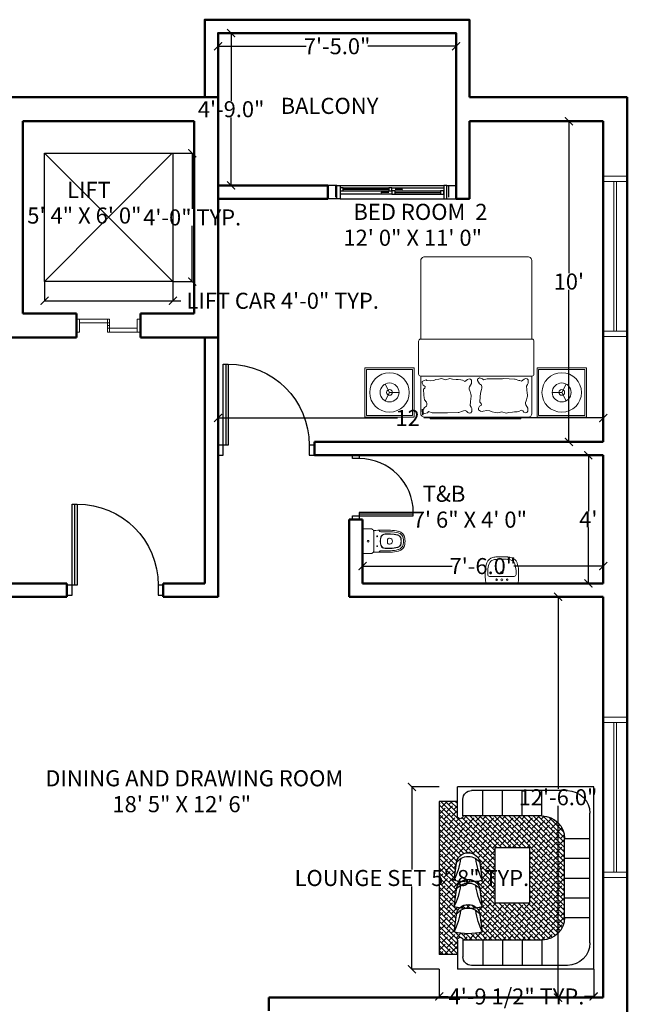
# Model space of a CAD drawing. Units: inches. Extents: x 147 to 1638, y 107 to 941.
# Tile 17 of 17: x 1368 to 1595, y 570 to 939. Entities that reach past the tile are written whole.
import ezdxf

# ---------------------------------------------------------------- set-up
doc = ezdxf.new("R2010")
doc.units = ezdxf.units.IN
doc.header["$MEASUREMENT"] = 0
for name, color, linetype, lineweight in [('A-ANNO-DIMS', 2, 'Continuous', 15), ('A-AREA-IDEN', 7, 'Continuous', 18), ('A-Door', 150, 'Continuous', 25), ('A-EQPM-ELEV', 7, 'Continuous', 25), ('A-FLOR-FIXT', 9, 'Continuous', 18), ('furniture', 50, 'Continuous', 18), ('HAT', 9, 'Continuous', 0), ('lift door', 200, 'Continuous', 20), ('walls', 7, 'Continuous', 50), ('windows', 3, 'Continuous', 20)]:
    doc.layers.add(name, color=color, linetype=linetype, lineweight=lineweight)
for name, color, linetype in [('A-Glaz', 92, 'Continuous'), ('FUR', 42, 'Continuous'), ('NT', 1, 'Continuous'), ('Win', 152, 'Continuous')]:
    doc.layers.add(name, color=color, linetype=linetype)
doc.styles.get("Standard").update_dxf_attribs({"font": 'arial.ttf'})
doc.dimstyles.get("Standard").update_dxf_attribs({"dimtxt": 6, "dimasz": 3, "dimexe": 0.18, "dimexo": 0.0625, "dimgap": 0.09, "dimtad": 0, "dimtih": 1, "dimtoh": 1, "dimdec": 1, "dimzin": 0, "dimdsep": 46, "dimlunit": 3, "dimtxsty": 'Standard', "dimblk": 'ARCHTICK', "dimcen": 0.09, "dimadec": 0, "dimazin": 0, "dimtfac": 1, "dimtdec": 1, "dimtofl": 0, "dimtmove": 0, "dimatfit": 3, "dimfxl": 1, "dimtolj": 1, "dimtzin": 0, "dimarcsym": 0})

# ---------------------------------------------------------------- blocks, each defined once
blk = doc.blocks.new('A$C087A3AA9')
at = {"layer": 'A-Door'}
for points in [[(852.6, 94.7), (852.6, 852.6), (805.3, 852.6), (805.3, 94.7)], [(47.4, 94.7), (47.4, 0), (0, 0), (0, 94.7)], [(900, 94.7), (900, 0), (852.6, 0), (852.6, 94.7)]]:
    blk.add_lwpolyline(points, close=True, dxfattribs=at)
at = {"layer": 'A-Glaz'}
blk.add_line((828.9, 852.6), (828.9, 94.7), dxfattribs=at)
at = {"layer": 'NT'}
blk.add_arc((805.3, 94.7), 757.9, 90, 180, dxfattribs=at)
blk = doc.blocks.new('_ArchTick')
at = {"color": 0, "linetype": 'ByBlock', "const_width": 0.15}
blk.add_lwpolyline([(-0.5, -0.5), (0.5, 0.5)], dxfattribs=at)
blk = doc.blocks.new('*D44')
at = {"layer": 'A-ANNO-DIMS', "color": 0, "lineweight": -2, "transparency": 16777216}
for p, q in [((1576.66, 722.72), (1568.7, 722.72)), ((1568.88, 722.72), (1568.88, 650.87)), ((1568.88, 572.72), (1568.88, 644.56)), ((1576.66, 572.72), (1568.7, 572.72))]:
    blk.add_line(p, q, dxfattribs=at)
at = {"layer": 'Defpoints', "color": 0, "lineweight": -2, "transparency": 16777216}
for p in [(1576.72, 722.72), (1568.88, 572.72), (1576.72, 572.72)]:
    blk.add_point(p, dxfattribs=at)
at = {"layer": 'A-ANNO-DIMS', "color": 0, "lineweight": -2, "transparency": 16777216, "xscale": 3, "yscale": 3, "zscale": 3}
for p, rotation in [((1568.88, 722.72), 90), ((1568.88, 572.72), 270)]:
    blk.add_blockref('_ArchTick', p, dxfattribs=dict(at, rotation=rotation))
at = {"layer": 'A-ANNO-DIMS', "color": 0, "transparency": 16777216, "insert": (1568.88, 647.72), "char_height": 6, "attachment_point": 5}
blk.add_mtext('\\A1;12\'-6.0"', dxfattribs=at)
blk = doc.blocks.new('*D45')
at = {"layer": 'A-ANNO-DIMS', "color": 0, "lineweight": -2, "transparency": 16777216}
for p, q in [((1566.15, 775.72), (1580.39, 775.72)), ((1580.21, 775.72), (1580.21, 754.81)), ((1580.21, 727.72), (1580.21, 748.63)), ((1566.15, 727.72), (1580.39, 727.72))]:
    blk.add_line(p, q, dxfattribs=at)
at = {"layer": 'Defpoints', "color": 0, "lineweight": -2, "transparency": 16777216}
for p in [(1566.09, 775.72), (1566.09, 727.72), (1580.21, 727.72)]:
    blk.add_point(p, dxfattribs=at)
at = {"layer": 'A-ANNO-DIMS', "color": 0, "lineweight": -2, "transparency": 16777216, "xscale": 3, "yscale": 3, "zscale": 3}
for p, rotation in [((1580.21, 775.72), 90), ((1580.21, 727.72), 270)]:
    blk.add_blockref('_ArchTick', p, dxfattribs=dict(at, rotation=rotation))
at = {"layer": 'A-ANNO-DIMS', "color": 0, "transparency": 16777216, "insert": (1580.21, 751.72), "char_height": 6, "attachment_point": 5}
blk.add_mtext("\\A1;4'", dxfattribs=at)
blk = doc.blocks.new('*D46')
at = {"layer": 'A-ANNO-DIMS', "color": 0, "lineweight": -2, "transparency": 16777216}
for p, q in [((1495.77, 730.37), (1495.77, 734.4)), ((1495.77, 734.22), (1529.23, 734.22)), ((1585.77, 734.22), (1552.3, 734.22)), ((1585.77, 730.37), (1585.77, 734.4))]:
    blk.add_line(p, q, dxfattribs=at)
at = {"layer": 'Defpoints', "color": 0, "lineweight": -2, "transparency": 16777216}
for p in [(1585.77, 734.22), (1495.77, 730.3), (1585.77, 730.3)]:
    blk.add_point(p, dxfattribs=at)
at = {"layer": 'A-ANNO-DIMS', "color": 0, "lineweight": -2, "transparency": 16777216, "xscale": 3, "yscale": 3, "zscale": 3, "rotation": 180}
blk.add_blockref('_ArchTick', (1495.77, 734.22), dxfattribs=at)
at = {"layer": 'A-ANNO-DIMS', "color": 0, "lineweight": -2, "transparency": 16777216, "xscale": 3, "yscale": 3, "zscale": 3}
blk.add_blockref('_ArchTick', (1585.77, 734.22), dxfattribs=at)
at = {"layer": 'A-ANNO-DIMS', "color": 0, "transparency": 16777216, "insert": (1540.77, 734.22), "char_height": 6, "attachment_point": 5}
blk.add_mtext('\\A1;7\'-6.0"', dxfattribs=at)
blk = doc.blocks.new('*D47')
at = {"layer": 'A-ANNO-DIMS', "color": 0, "lineweight": -2, "transparency": 16777216}
for p, q in [((1441.77, 785.96), (1441.77, 789.84)), ((1441.77, 789.66), (1508.87, 789.66)), ((1585.77, 789.66), (1518.67, 789.66)), ((1585.77, 785.96), (1585.77, 789.84))]:
    blk.add_line(p, q, dxfattribs=at)
at = {"layer": 'Defpoints', "color": 0, "lineweight": -2, "transparency": 16777216}
for p in [(1585.77, 789.66), (1441.77, 785.9), (1585.77, 785.9)]:
    blk.add_point(p, dxfattribs=at)
at = {"layer": 'A-ANNO-DIMS', "color": 0, "lineweight": -2, "transparency": 16777216, "xscale": 3, "yscale": 3, "zscale": 3, "rotation": 180}
blk.add_blockref('_ArchTick', (1441.77, 789.66), dxfattribs=at)
at = {"layer": 'A-ANNO-DIMS', "color": 0, "lineweight": -2, "transparency": 16777216, "xscale": 3, "yscale": 3, "zscale": 3}
blk.add_blockref('_ArchTick', (1585.77, 789.66), dxfattribs=at)
at = {"layer": 'A-ANNO-DIMS', "color": 0, "transparency": 16777216, "insert": (1513.77, 789.66), "char_height": 6, "attachment_point": 5}
blk.add_mtext("\\A1;12'", dxfattribs=at)
blk = doc.blocks.new('*D48')
at = {"layer": 'A-ANNO-DIMS', "color": 0, "lineweight": -2, "transparency": 16777216}
for p, q in [((1578.32, 900.72), (1572.74, 900.72)), ((1572.92, 900.72), (1572.92, 843.87)), ((1572.92, 780.72), (1572.92, 837.56)), ((1578.32, 780.72), (1572.74, 780.72))]:
    blk.add_line(p, q, dxfattribs=at)
at = {"layer": 'Defpoints', "color": 0, "lineweight": -2, "transparency": 16777216}
for p in [(1578.38, 900.72), (1572.92, 780.72), (1578.38, 780.72)]:
    blk.add_point(p, dxfattribs=at)
at = {"layer": 'A-ANNO-DIMS', "color": 0, "lineweight": -2, "transparency": 16777216, "xscale": 3, "yscale": 3, "zscale": 3}
for p, rotation in [((1572.92, 900.72), 90), ((1572.92, 780.72), 270)]:
    blk.add_blockref('_ArchTick', p, dxfattribs=dict(at, rotation=rotation))
at = {"layer": 'A-ANNO-DIMS', "color": 0, "transparency": 16777216, "insert": (1572.92, 840.72), "char_height": 6, "attachment_point": 5}
blk.add_mtext("\\A1;10'", dxfattribs=at)
blk = doc.blocks.new('*D53')
at = {"layer": 'A-ANNO-DIMS', "color": 0, "lineweight": -2, "transparency": 16777216}
for p, q in [((1441.77, 928.85), (1441.77, 928.97)), ((1441.77, 928.79), (1474.73, 928.79)), ((1530.77, 928.79), (1497.8, 928.79)), ((1530.77, 928.85), (1530.77, 928.97))]:
    blk.add_line(p, q, dxfattribs=at)
at = {"layer": 'Defpoints', "color": 0, "lineweight": -2, "transparency": 16777216}
for p in [(1441.77, 928.79), (1530.77, 928.79), (1530.77, 928.79)]:
    blk.add_point(p, dxfattribs=at)
at = {"layer": 'A-ANNO-DIMS', "color": 0, "lineweight": -2, "transparency": 16777216, "xscale": 3, "yscale": 3, "zscale": 3, "rotation": 180}
blk.add_blockref('_ArchTick', (1441.77, 928.79), dxfattribs=at)
at = {"layer": 'A-ANNO-DIMS', "color": 0, "lineweight": -2, "transparency": 16777216, "xscale": 3, "yscale": 3, "zscale": 3}
blk.add_blockref('_ArchTick', (1530.77, 928.79), dxfattribs=at)
at = {"layer": 'A-ANNO-DIMS', "color": 0, "transparency": 16777216, "insert": (1486.27, 928.79), "char_height": 6, "attachment_point": 5}
blk.add_mtext('\\A1;7\'-5.0"', dxfattribs=at)
blk = doc.blocks.new('*D54')
at = {"layer": 'A-ANNO-DIMS', "color": 0, "lineweight": -2, "transparency": 16777216}
for p, q in [((1446.17, 933.72), (1446.83, 933.72)), ((1446.65, 933.72), (1446.65, 908.37)), ((1446.65, 876.72), (1446.65, 902.06)), ((1446.17, 876.72), (1446.83, 876.72))]:
    blk.add_line(p, q, dxfattribs=at)
at = {"layer": 'Defpoints', "color": 0, "lineweight": -2, "transparency": 16777216}
for p in [(1446.11, 933.72), (1446.11, 876.72), (1446.65, 876.72)]:
    blk.add_point(p, dxfattribs=at)
at = {"layer": 'A-ANNO-DIMS', "color": 0, "lineweight": -2, "transparency": 16777216, "xscale": 3, "yscale": 3, "zscale": 3}
for p, rotation in [((1446.65, 933.72), 90), ((1446.65, 876.72), 270)]:
    blk.add_blockref('_ArchTick', p, dxfattribs=dict(at, rotation=rotation))
at = {"layer": 'A-ANNO-DIMS', "color": 0, "transparency": 16777216, "insert": (1446.65, 905.22), "char_height": 6, "attachment_point": 5}
blk.add_mtext('\\A1;4\'-9.0"', dxfattribs=at)
blk = doc.blocks.new('MAT-P14')
for p, q in [((-1.337, 1.348), (-1.337, 1.948)), ((-1.337, 1.948), (-0.737, 1.948)), ((-1.317, 1.928), (-0.757, 1.928)), ((-1.317, 1.368), (-1.317, 1.928)), ((-0.757, 1.368), (-0.757, 1.928)), ((-0.737, 1.348), (-0.737, 1.948)), ((0.625, 1.95), (-0.625, 1.95)), ((0.753, 1.348), (0.753, 1.948)), ((1.353, 1.948), (0.753, 1.948)), ((1.333, 1.928), (0.773, 1.928)), ((0.773, 1.368), (0.773, 1.928)), ((1.333, 1.368), (1.333, 1.928)), ((1.353, 1.348), (1.353, 1.948)), ((-1.037, 1.648), (-1.091, 1.749)), ((1.053, 1.648), (1.108, 1.749)), ((-1.037, 1.648), (-1.091, 1.547)), ((-1.037, 1.648), (-0.922, 1.648)), ((1.053, 1.648), (0.938, 1.648)), ((1.053, 1.648), (1.108, 1.547)), ((-1.337, 1.348), (-0.737, 1.348)), ((-1.317, 1.368), (-0.757, 1.368)), ((1.353, 1.348), (0.753, 1.348)), ((1.333, 1.368), (0.773, 1.368))]:
    blk.add_line(p, q)
for points in [[(-0.675, 1.45), (-0.675, 1.9, -0.414214), (-0.625, 1.95), (0.625, 1.95, -0.414214), (0.675, 1.9), (0.675, 1.45)], [(-0.675, 1, -0.414214), (-0.7, 1.025), (-0.7, 1.425, -0.414214), (-0.675, 1.45), (0.675, 1.45, -0.414214), (0.7, 1.425), (0.7, 1.025, -0.414214), (0.675, 1)], [(-0.625, 0, -0.414214), (-0.675, 0.05), (-0.675, 1), (0.675, 1), (0.675, 0.05, -0.414214), (0.625, 0)]]:
    blk.add_lwpolyline(points, format="xyb", close=True)
blk.add_lwpolyline([(-0.542, 1.95), (-0.542, 1.967), (0.558, 1.967), (0.558, 1.95)], close=True)
for points in [[(-0.614, 1.818), (-0.626, 1.838), (-0.626, 1.877), (-0.614, 1.891), (-0.596, 1.896), (-0.579, 1.886), (-0.563, 1.872), (-0.545, 1.863), (-0.516, 1.879), (-0.497, 1.882), (-0.465, 1.884), (-0.439, 1.887), (-0.395, 1.892), (-0.363, 1.9), (-0.309, 1.882), (-0.262, 1.897), (-0.23, 1.892), (-0.192, 1.884), (-0.166, 1.873), (-0.128, 1.868), (-0.082, 1.875), (-0.076, 1.88), (-0.052, 1.875), (-0.028, 1.861), (-0.028, 1.841), (-0.04, 1.817), (-0.064, 1.802), (-0.06, 1.781), (-0.043, 1.768), (-0.046, 1.697), (-0.05, 1.662), (-0.056, 1.64), (-0.062, 1.612), (-0.068, 1.596), (-0.068, 1.579), (-0.063, 1.56), (-0.039, 1.545), (-0.015, 1.505), (-0.015, 1.486), (-0.038, 1.471), (-0.075, 1.482), (-0.081, 1.487), (-0.087, 1.497), (-0.134, 1.481), (-0.304, 1.482), (-0.318, 1.482), (-0.335, 1.479), (-0.464, 1.488), (-0.467, 1.486), (-0.473, 1.486), (-0.517, 1.503), (-0.53, 1.505), (-0.548, 1.51), (-0.566, 1.501), (-0.581, 1.487), (-0.599, 1.477), (-0.617, 1.482), (-0.629, 1.497), (-0.629, 1.536), (-0.623, 1.55), (-0.611, 1.57), (-0.614, 1.614), (-0.615, 1.627), (-0.618, 1.644), (-0.619, 1.66), (-0.62, 1.675), (-0.62, 1.695), (-0.618, 1.707), (-0.614, 1.723), (-0.608, 1.739), (-0.604, 1.75), (-0.598, 1.771), (-0.596, 1.785), (-0.6, 1.798), (-0.614, 1.819)], [(0.069, 1.559), (0.057, 1.54), (0.057, 1.501), (0.069, 1.486), (0.087, 1.481), (0.105, 1.491), (0.121, 1.505), (0.139, 1.514), (0.168, 1.498), (0.187, 1.496), (0.219, 1.493), (0.244, 1.49), (0.289, 1.485), (0.321, 1.477), (0.374, 1.495), (0.422, 1.48), (0.454, 1.486), (0.492, 1.493), (0.517, 1.504), (0.555, 1.509), (0.602, 1.502), (0.608, 1.497), (0.632, 1.502), (0.656, 1.517), (0.656, 1.536), (0.644, 1.561), (0.62, 1.575), (0.624, 1.596), (0.641, 1.609), (0.637, 1.68), (0.633, 1.715), (0.628, 1.738), (0.606, 1.765), (0.6, 1.781), (0.6, 1.798), (0.605, 1.817), (0.629, 1.832), (0.654, 1.872), (0.654, 1.892), (0.63, 1.906), (0.593, 1.895), (0.587, 1.891), (0.581, 1.881), (0.534, 1.896), (0.379, 1.896), (0.366, 1.896), (0.348, 1.898), (0.22, 1.89), (0.216, 1.891), (0.21, 1.891), (0.167, 1.875), (0.154, 1.872), (0.136, 1.867), (0.118, 1.876), (0.102, 1.89), (0.085, 1.9), (0.067, 1.895), (0.055, 1.881), (0.055, 1.842), (0.061, 1.827), (0.073, 1.807), (0.07, 1.764), (0.069, 1.75), (0.066, 1.733), (0.065, 1.718), (0.063, 1.703), (0.063, 1.682), (0.066, 1.67), (0.07, 1.655), (0.075, 1.638), (0.079, 1.627), (0.086, 1.607), (0.087, 1.592), (0.083, 1.579), (0.07, 1.559)]]:
    blk.add_lwpolyline(points)
for centre, radius in [((-1.037, 1.648), 0.24), ((1.053, 1.648), 0.24), ((-1.037, 1.648), 0.115), ((-1.037, 1.648), 0.035), ((1.053, 1.648), 0.115), ((1.053, 1.648), 0.035)]:
    blk.add_circle(centre, radius)
blk = doc.blocks.new('2SAINDA')
at = {"color": 0, "linetype": 'ByBlock'}
for p, q in [((0, 0.188), (0, -0.188)), ((0.018, 0.2), (0.141, 0.2)), ((0.157, 0.192), (0.162, 0.188)), ((0.18, -0.164), (0.18, 0.164)), ((0.279, 0.159), (0.261, 0.176)), ((0.437, 0.047), (0.424, 0.047)), ((0.279, -0.159), (0.261, -0.176)), ((0.437, -0.047), (0.424, -0.047)), ((0.018, -0.2), (0.141, -0.2)), ((0.157, -0.192), (0.162, -0.188))]:
    blk.add_line(p, q, dxfattribs=at)
for centre, radius in [((0.09, 0), 0.0135), ((0.09, 0), 0.0135), ((0.236, 0.08), 0.0075), ((0.236, -0.08), 0.0075)]:
    blk.add_circle(centre, radius, dxfattribs=at)
for centre, radius, start, end in [((0.018, 0.18), 0.02, 90, 155.6901), ((0.141, 0.181), 0.019, 34.9372, 90), ((0.155, 0.164), 0.025, 23.3776, 73.7848), ((0.383, -5.322), 5.5, 89.2905, 92.1362), ((0.155, 0.164), 0.025, 360, 23.3776), ((0.444, -0.373), 0.55, 75.4605, 89.2905), ((0.549, 0.03), 0.134, 8.8162, 75.4605), ((0.293, 0.173), 0.02, 225, 270.9364), ((0.485, 0), 0.2, 160.016, 199.984), ((0.485, 0), 0.196, 160.016, 199.984), ((0.383, -5.322), 5.476, 89.2905, 90.9364), ((0.368, 0.043), 0.075, 90.1648, 160.016), ((0.368, 0.043), 0.071, 90.1648, 160.016), ((0.383, -5.322), 5.44, 89.2905, 90.1648), ((0.383, -5.322), 5.436, 89.2905, 90.1648), ((0.582, 0), 0.18, 170.2849, 189.7151), ((0.424, 0.027), 0.02, 90, 170.2849), ((0.437, 0), 0.047, 0, 90), ((0.437, 0), 0.047, 270, 0), ((0.444, -0.373), 0.49, 75.4605, 89.2905), ((0.444, -0.373), 0.486, 75.4605, 89.2905), ((0.444, -0.373), 0.526, 75.4605, 89.2905), ((0.549, 0.03), 0.07, 8.8162, 75.4605), ((0.549, 0.03), 0.074, 8.8162, 75.4605), ((0.549, 0.03), 0.11, 8.8162, 75.4605), ((0.355, 0), 0.266, 351.1838, 8.8162), ((0.355, 0), 0.27, 351.1838, 8.8162), ((0.355, 0), 0.306, 351.1838, 8.8162), ((0.355, 0), 0.33, 351.1838, 8.8162), ((0.293, -0.173), 0.02, 89.0636, 135), ((0.383, 5.322), 5.476, 269.0636, 270.7095), ((0.368, -0.043), 0.075, 199.984, 269.8352), ((0.368, -0.043), 0.071, 199.984, 269.8352), ((0.383, 5.322), 5.436, 269.8352, 270.7095), ((0.383, 5.322), 5.44, 269.8352, 270.7095), ((0.424, -0.027), 0.02, 189.7151, 270), ((0.444, 0.373), 0.486, 270.7095, 284.5395), ((0.444, 0.373), 0.49, 270.7095, 284.5395), ((0.444, 0.373), 0.526, 270.7095, 284.5395), ((0.549, -0.03), 0.07, 284.5395, 351.1838), ((0.549, -0.03), 0.074, 284.5395, 351.1838), ((0.549, -0.03), 0.11, 284.5395, 351.1838), ((0.549, -0.03), 0.134, 284.5395, 351.1838), ((0.018, -0.18), 0.02, 204.3099, 270), ((0.141, -0.181), 0.019, 270, 325.0628), ((0.155, -0.164), 0.025, 286.2152, 336.6224), ((0.155, -0.164), 0.025, 336.6224, 0), ((0.383, 5.322), 5.5, 267.8638, 270.7095), ((0.444, 0.373), 0.55, 270.7095, 284.5395)]:
    blk.add_arc(centre, radius, start, end, dxfattribs=at)
blk = doc.blocks.new('2SALADA2')
at = {"color": 0}
for p, q in [((-0.296, 0), (0.296, 0)), ((0.207, -0.13), (-0.207, -0.13))]:
    blk.add_line(p, q, dxfattribs=at)
for centre, radius in [((-0.1, -0.07), 0.015), ((0, -0.205), 0.023), ((0, -0.07), 0.0175), ((0.1, -0.07), 0.015)]:
    blk.add_circle(centre, radius, dxfattribs=at)
for centre, radius, start, end in [((-0.296, -0.01), 0.01, 90, 173.6262), ((0.296, -0.01), 0.01, 6.3738, 90), ((1.185, -0.175), 1.5, 173.6262, 182.693), ((1.186, -0.221), 1.454, 178.0234, 180.898), ((-0.227, -0.171), 0.04, 95.5937, 179.6995), ((-0.207, -0.38), 0.25, 90, 95.5937), ((0.207, -0.38), 0.25, 84.4063, 90), ((0.227, -0.171), 0.04, 0.3005, 84.4063), ((-1.186, -0.221), 1.454, 359.102, 1.9766), ((-1.185, -0.175), 1.5, 357.307, 6.3738), ((0.186, -0.222), 0.5, 182.693, 199.3406), ((0.186, -0.222), 0.454, 182.693, 199.3406), ((-0.186, -0.222), 0.454, 340.6594, 357.307), ((-0.186, -0.222), 0.5, 340.6594, 357.307), ((-0.135, -0.335), 0.16, 199.3406, 257.4429), ((-0.135, -0.335), 0.114, 199.3406, 257.4429), ((-0.061, -0.003), 0.5, 257.4429, 266.4982), ((-0.061, -0.003), 0.454, 257.4429, 266.4982), ((0, 0.995), 1.5, 266.4982, 273.5018), ((0, 0.995), 1.454, 266.4982, 273.5018), ((0.061, -0.003), 0.454, 273.5018, 282.5571), ((0.061, -0.003), 0.5, 273.5018, 282.5571), ((0.135, -0.335), 0.114, 282.5571, 340.6594), ((0.135, -0.335), 0.16, 282.5571, 340.6594)]:
    blk.add_arc(centre, radius, start, end, dxfattribs=at)
blk = doc.blocks.new('CHAIR1')
for p, q in [((-393, -750), (-329, -287)), ((329, -286), (394, -750))]:
    blk.add_line(p, q)
for centre, radius, start, end in [((0, -332), 332, 7.9072, 172.1612), ((-1856, 27), 1657, 332.0394, 353.4161), ((0, -483), 383, 30.9021, 149.1663), ((1857, 27), 1657, 186.5839, 207.9606), ((0, 770), 1570, 255.502, 284.498)]:
    blk.add_arc(centre, radius, start, end)
blk = doc.blocks.new('A$C1CFC4E3A')
at = {"layer": 'HAT'}
h = blk.add_hatch(dxfattribs=at)
h.set_pattern_fill('ANSI38,_O', color=256, scale=0.664121)
h.set_pattern_definition([(45, (6.13299, -18.48134), (-0.05870057, 0.05870057), []), (135, (6.13299, -18.48134), (-0.1761017, 0.05870057), [0.2075378, -0.1245227])])
h.paths.add_polyline_path([(0, 3.705), (-0.438, 3.705), (-0.438, 3.353, -1), (-0.573, 3.353), (-2.482, 3.353, 0.414214), (-3.028, 2.807), (-3.028, 0.898, 0.414214), (-2.482, 0.352), (-0.573, 0.352, -1), (-0.438, 0.352), (-0.438, 0), (0, 0)])
h.paths.add_polyline_path([(-1.342, 1.248), (-2.191, 1.248), (-2.191, 2.58), (-1.342, 2.58)], flags=16)
h.paths.add_polyline_path([(-0.409, 1.566), (-0.352, 1.156, -0.127199), (-1.048, 1.156), (-0.992, 1.566, -0.871235)], flags=16)
h.paths.add_polyline_path([(-0.409, 0.959), (-0.352, 0.548, -0.127199), (-1.048, 0.548), (-0.992, 0.958, -0.871235)], flags=16)
h.paths.add_polyline_path([(-0.992, 2.209, -0.871235), (-0.409, 2.21), (-0.352, 1.799, -0.127199), (-1.048, 1.799)], flags=16)
at = {"layer": 'FUR'}
for p, q in [((-3.732, 4.057), (-0.438, 4.057)), ((-3.732, -0.352), (-3.732, 4.057)), ((-0.438, 3.353), (-0.438, 4.057)), ((-3.096, 3.967), (-0.777, 3.967)), ((-2.482, 3.353), (-2.482, 3.967)), ((-2.005, 3.353), (-2.005, 3.967)), ((-1.528, 3.353), (-1.528, 3.967)), ((-1.05, 3.353), (-1.05, 3.967)), ((-0.573, 3.353), (-0.573, 3.762)), ((-3.642, 0.284), (-3.642, 3.421)), ((-2.482, 3.353), (-0.573, 3.353)), ((-3.028, 2.807), (-3.642, 2.807)), ((-3.028, 2.33), (-3.642, 2.33)), ((-3.028, 1.852), (-3.642, 1.852)), ((-3.028, 1.375), (-3.642, 1.375)), ((-3.028, 0.898), (-3.642, 0.898)), ((-2.482, 0.352), (-0.573, 0.352)), ((-2.482, 0.352), (-2.482, -0.262)), ((-2.005, 0.352), (-2.005, -0.262)), ((-1.528, 0.352), (-1.528, -0.262)), ((-1.05, 0.352), (-1.05, -0.262)), ((-0.573, 0.352), (-0.573, -0.057)), ((-0.438, 0.352), (-0.438, -0.352)), ((-3.732, -0.352), (-0.438, -0.352)), ((-3.096, -0.262), (-0.777, -0.262))]:
    blk.add_line(p, q, dxfattribs=at)
for centre, radius, start, end in [((-3.096, 3.421), 0.546, 90, 180), ((-0.777, 3.762), 0.205, 0, 90), ((-2.482, 2.807), 0.546, 90, 180), ((-0.505, 3.353), 0.0675, 180, 0), ((-2.482, 0.898), 0.546, 180, 270), ((-3.096, 0.284), 0.546, 180, 270), ((-0.505, 0.352), 0.0675, 0, 180), ((-0.777, -0.057), 0.205, 270, 0)]:
    blk.add_arc(centre, radius, start, end, dxfattribs=at)
at = {"layer": 'Win'}
for p, q in [((-0.438, 3.705), (0, 3.705)), ((0, 3.705), (0, 0)), ((-3.028, 0.898), (-3.028, 2.807)), ((-0.438, 0), (0, 0))]:
    blk.add_line(p, q, dxfattribs=at)
blk.add_lwpolyline([(-2.191, 2.58), (-1.342, 2.58), (-1.342, 1.248), (-2.191, 1.248)], close=True, dxfattribs=at)
at = {"layer": 'FUR', "xscale": 0.0008854948152227, "yscale": 0.0008854948152227, "zscale": 0.0008854948152227}
for p in [(-0.7, 2.463), (-0.7, 1.82), (-0.7, 1.212)]:
    blk.add_blockref('CHAIR1', p, dxfattribs=at)
blk = doc.blocks.new('WIN-60IN')
for p, q in [((60, 9), (0, 9)), ((0, 9), (0, 0)), ((2, 9), (2, 0)), ((58, 0), (58, 9)), ((60, 0), (60, 9)), ((2, 5), (58, 5)), ((2, 4), (58, 4)), ((0, 0), (60, 0))]:
    blk.add_line(p, q)
blk = doc.blocks.new('DOOR-SLIDING-48IN')
for p, q in [((3.46, 5), (0, 5)), ((2.87, 5), (2.87, 0.59)), ((3.46, 0), (3.46, 5)), ((3.46, 5), (4.63, 5)), ((4.63, 5), (43.37, 5)), ((4.63, 5), (4.63, 0)), ((5.81, 4.11), (22.83, 4.11)), ((24, 4.11), (43.37, 4.11)), ((44.54, 5), (43.37, 5)), ((43.37, 5), (43.37, 0)), ((44.54, 5), (48, 5)), ((44.54, 0), (44.54, 5)), ((45.13, 5), (45.13, 0.59)), ((3.46, 0), (0, 0)), ((4.63, 0), (3.46, 0)), ((24, 1.76), (4.63, 1.76)), ((4.63, 0), (43.37, 0)), ((5.81, 3.52), (22.83, 3.52)), ((5.81, 2.93), (22.83, 2.93)), ((22.83, 2.35), (20.3, 2.35)), ((25.17, 3.52), (27.7, 3.52)), ((25.17, 2.93), (42.19, 2.93)), ((25.17, 2.35), (42.19, 2.35)), ((25.17, 1.76), (42.19, 1.76)), ((43.37, 0), (44.54, 0)), ((44.54, 0), (48, 0))]:
    blk.add_line(p, q)
for points in [[(4.63, 2.93), (5.81, 2.93), (5.81, 4.11), (4.63, 4.11)], [(22.83, 2.93), (24, 2.93), (24, 4.11), (22.83, 4.11)], [(28, 3.52), (27.7, 3.7), (27.7, 3.35)], [(20, 2.35), (20.3, 2.52), (20.3, 2.17)], [(24, 1.76), (25.17, 1.76), (25.17, 2.93), (24, 2.93)], [(42.19, 1.76), (43.37, 1.76), (43.37, 2.93), (42.19, 2.93)]]:
    blk.add_lwpolyline(points, close=True)
blk = doc.blocks.new('LIFT-CAR')
for p, q in [((48, 0), (0, 48)), ((47.77, 48), (0, 0))]:
    blk.add_line(p, q)
blk.add_lwpolyline([(0, 48), (48, 48), (48, 0), (0, 0)], close=True)
blk = doc.blocks.new('LIFT-DOOR-CENTER-OPEN')
for p, q in [((1.24, 4.95), (12.38, 4.95)), ((11.62, 2.48), (11.62, 4.95)), ((12.38, 4.95), (12.38, 2.48)), ((1.24, 3.49), (12.38, 3.49)), ((11.62, 0), (11.62, 2.48)), ((11.62, 2.48), (12.38, 2.48)), ((12.38, 2.48), (11.62, 2.48)), ((22.76, 1.47), (11.62, 1.47)), ((12.38, 2.48), (12.38, 0)), ((22.76, 0), (11.62, 0))]:
    blk.add_line(p, q)
for points in [[(1.24, 0), (0, 0), (0, 4.95), (1.24, 4.95)], [(22.76, 4.95), (24, 4.95), (24, 0), (22.76, 0)]]:
    blk.add_lwpolyline(points, close=True)
blk = doc.blocks.new('*D112')
at = {"layer": 'A-ANNO-DIMS', "color": 0, "lineweight": -2, "transparency": 16777216}
for p, q in [((1524.4, 651.59), (1514.05, 651.59)), ((1514.23, 651.59), (1514.23, 620.68)), ((1514.23, 583.38), (1514.23, 614.29)), ((1524.4, 583.38), (1514.05, 583.38))]:
    blk.add_line(p, q, dxfattribs=at)
at = {"layer": 'Defpoints', "color": 0, "lineweight": -2, "transparency": 16777216}
for p in [(1514.23, 651.59), (1524.46, 651.59), (1524.46, 583.38)]:
    blk.add_point(p, dxfattribs=at)
at = {"layer": 'A-ANNO-DIMS', "color": 0, "lineweight": -2, "transparency": 16777216, "xscale": 3, "yscale": 3, "zscale": 3}
for p, rotation in [((1514.23, 651.59), 90), ((1514.23, 583.38), 270)]:
    blk.add_blockref('_ArchTick', p, dxfattribs=dict(at, rotation=rotation))
at = {"layer": 'A-ANNO-DIMS', "color": 0, "transparency": 16777216, "insert": (1514.23, 617.49), "char_height": 6, "attachment_point": 5}
blk.add_mtext('\\A1;LOUNGE SET 5\'-8" TYP.', dxfattribs=at)
blk = doc.blocks.new('*D113')
at = {"layer": 'A-ANNO-DIMS', "color": 0, "lineweight": -2, "transparency": 16777216}
for p, q in [((1524.46, 583.32), (1524.46, 572.97)), ((1582.2, 583.32), (1582.2, 572.97)), ((1524.46, 573.15), (1527.84, 573.15)), ((1582.2, 573.15), (1578.82, 573.15))]:
    blk.add_line(p, q, dxfattribs=at)
at = {"layer": 'Defpoints', "color": 0, "lineweight": -2, "transparency": 16777216}
for p in [(1524.46, 583.38), (1582.2, 583.38), (1524.46, 573.15)]:
    blk.add_point(p, dxfattribs=at)
at = {"layer": 'A-ANNO-DIMS', "color": 0, "lineweight": -2, "transparency": 16777216, "xscale": 3, "yscale": 3, "zscale": 3, "rotation": 180}
blk.add_blockref('_ArchTick', (1524.46, 573.15), dxfattribs=at)
at = {"layer": 'A-ANNO-DIMS', "color": 0, "lineweight": -2, "transparency": 16777216, "xscale": 3, "yscale": 3, "zscale": 3}
blk.add_blockref('_ArchTick', (1582.2, 573.15), dxfattribs=at)
at = {"layer": 'A-ANNO-DIMS', "color": 0, "transparency": 16777216, "insert": (1553.33, 573.15), "char_height": 6, "attachment_point": 5}
blk.add_mtext('\\A1;4\'-9 1/2" TYP.', dxfattribs=at)
blk = doc.blocks.new('*D128')
at = {"layer": 'A-ANNO-DIMS', "color": 0, "lineweight": -2, "transparency": 16777216}
for p, q in [((1376.88, 840.66), (1376.88, 833.34)), ((1424.88, 840.66), (1424.88, 833.34)), ((1376.88, 833.52), (1424.88, 833.52)), ((1424.88, 833.52), (1427.88, 833.52))]:
    blk.add_line(p, q, dxfattribs=at)
at = {"layer": 'Defpoints', "color": 0, "lineweight": -2, "transparency": 16777216}
for p in [(1376.88, 840.72), (1424.88, 840.72), (1424.88, 833.52)]:
    blk.add_point(p, dxfattribs=at)
at = {"layer": 'A-ANNO-DIMS', "color": 0, "lineweight": -2, "transparency": 16777216, "xscale": 3, "yscale": 3, "zscale": 3, "rotation": 180}
blk.add_blockref('_ArchTick', (1376.88, 833.52), dxfattribs=at)
at = {"layer": 'A-ANNO-DIMS', "color": 0, "lineweight": -2, "transparency": 16777216, "xscale": 3, "yscale": 3, "zscale": 3}
blk.add_blockref('_ArchTick', (1424.88, 833.52), dxfattribs=at)
at = {"layer": 'A-ANNO-DIMS', "color": 0, "transparency": 16777216, "insert": (1465.92, 833.52), "char_height": 6, "attachment_point": 5}
blk.add_mtext('\\A1;LIFT CAR 4\'-0" TYP.', dxfattribs=at)
blk = doc.blocks.new('*D129')
at = {"layer": 'A-ANNO-DIMS', "color": 0, "lineweight": -2, "transparency": 16777216}
for p, q in [((1424.94, 888.72), (1432.26, 888.72)), ((1432.08, 888.72), (1432.08, 867.87)), ((1432.08, 840.72), (1432.08, 861.57)), ((1424.94, 840.72), (1432.26, 840.72))]:
    blk.add_line(p, q, dxfattribs=at)
at = {"layer": 'Defpoints', "color": 0, "lineweight": -2, "transparency": 16777216}
for p in [(1424.88, 888.72), (1432.08, 888.72), (1424.88, 840.72)]:
    blk.add_point(p, dxfattribs=at)
at = {"layer": 'A-ANNO-DIMS', "color": 0, "lineweight": -2, "transparency": 16777216, "xscale": 3, "yscale": 3, "zscale": 3}
for p, rotation in [((1432.08, 888.72), 90), ((1432.08, 840.72), 270)]:
    blk.add_blockref('_ArchTick', p, dxfattribs=dict(at, rotation=rotation))
at = {"layer": 'A-ANNO-DIMS', "color": 0, "transparency": 16777216, "insert": (1432.08, 864.72), "char_height": 6, "attachment_point": 5}
blk.add_mtext('\\A1;4\'-0" TYP.', dxfattribs=at)

msp = doc.modelspace()

# ---------------------------------------------------------------- linework, layer by layer
at = {"layer": 'walls'}
for p, q in [((1270.77, 909.72), (1441.77, 909.72)), ((1441.77, 909.72), (1441.77, 780.72)), ((1535.77, 909.72), (1594.77, 909.72)), ((1594.77, 909.72), (1594.77, 201.72)), ((1368.77, 900.72), (1368.77, 828.72)), ((1368.77, 900.72), (1432.77, 900.72)), ((1432.77, 900.72), (1432.77, 828.72)), ((1535.77, 900.72), (1585.77, 900.72)), ((1585.77, 900.72), (1585.77, 780.72)), ((1482.77, 876.72), (1482.77, 871.72)), ((1530.77, 876.72), (1530.77, 871.72)), ((1368.77, 828.72), (1388.77, 828.72)), ((1388.77, 828.72), (1388.77, 819.72)), ((1412.77, 828.72), (1432.77, 828.72)), ((1412.77, 828.72), (1412.77, 819.72)), ((1359.77, 819.72), (1388.77, 819.72)), ((1412.77, 819.72), (1441.77, 819.72)), ((1436.77, 819.72), (1436.77, 727.72)), ((1441.77, 775.72), (1441.77, 780.72)), ((1477.77, 780.72), (1585.77, 780.72)), ((1477.77, 775.72), (1477.77, 780.72)), ((1441.77, 775.72), (1441.77, 722.72)), ((1477.77, 775.72), (1490.77, 775.72)), ((1490.77, 775.72), (1495.77, 775.72)), ((1495.77, 775.72), (1585.77, 775.72)), ((1585.77, 775.72), (1585.77, 727.72)), ((1490.77, 751.72), (1490.77, 722.72)), ((1490.77, 751.72), (1495.77, 751.72)), ((1495.77, 751.72), (1495.77, 727.72)), ((1333.27, 727.72), (1385.27, 727.72)), ((1385.27, 722.72), (1385.27, 727.72)), ((1421.27, 727.72), (1436.77, 727.72)), ((1421.27, 722.72), (1421.27, 727.72)), ((1495.77, 727.72), (1585.77, 727.72)), ((1364.77, 722.72), (1385.27, 722.72)), ((1421.27, 722.72), (1441.77, 722.72)), ((1490.77, 722.72), (1585.77, 722.72)), ((1585.77, 722.72), (1585.77, 572.72)), ((1460.77, 572.72), (1460.77, 567.72)), ((1460.77, 572.72), (1585.77, 572.72))]:
    msp.add_line(p, q, dxfattribs=at)
for points in [[(1436.77, 909.72), (1436.77, 938.72), (1535.77, 938.72), (1535.77, 909.72)], [(1441.77, 909.72), (1441.77, 933.72), (1530.77, 933.72), (1530.77, 909.72)], [(1530.77, 909.72), (1530.77, 876.72)], [(1535.77, 900.72), (1535.77, 871.72), (1530.77, 871.72)], [(1482.77, 876.72), (1441.77, 876.72)], [(1482.77, 871.72), (1441.77, 871.72)]]:
    msp.add_lwpolyline(points, dxfattribs=at)

# ---------------------------------------------------------------- block references
at = {"layer": 'A-Door'}
msp.add_blockref('DOOR-SLIDING-48IN', (1482.77, 871.72), dxfattribs=at)
at = {"layer": 'A-Door', "xscale": -0.0400000000000001, "yscale": 0.0400000000000001, "zscale": 0.0400000000000001}
for p in [(1477.77, 775.72), (1421.27, 723.32)]:
    msp.add_blockref('A$C087A3AA9', p, dxfattribs=at)
at = {"layer": 'A-Door', "xscale": 0.0266666667542921, "yscale": 0.0266666667542921, "zscale": 0.0266666667542921, "rotation": 270}
msp.add_blockref('A$C087A3AA9', (1492.03, 775.72), dxfattribs=at)
at = {"layer": 'A-EQPM-ELEV'}
msp.add_blockref('LIFT-CAR', (1376.88, 840.72), dxfattribs=at)
at = {"layer": 'A-FLOR-FIXT', "xscale": 23.19012112898009, "yscale": 23.19012112898009, "zscale": 23.19012112898009}
msp.add_blockref('2SAINDA', (1495.77, 743.53), dxfattribs=at)
at = {"layer": 'A-FLOR-FIXT', "xscale": 19.81841434140962, "yscale": 19.81841434140962, "zscale": 19.81841434140962, "rotation": 180}
msp.add_blockref('2SALADA2', (1547.88, 727.72), dxfattribs=at)
at = {"layer": 'furniture', "xscale": 30.80045642108221, "yscale": 30.80045642108221, "zscale": 30.80045642108221, "rotation": 180}
msp.add_blockref('MAT-P14', (1538.31, 849.98), dxfattribs=at)
at = {"layer": 'furniture', "xscale": -15.47145176415956, "yscale": 15.47145176415956, "zscale": 15.47145176415956}
msp.add_blockref('A$C1CFC4E3A', (1524.46, 588.83), dxfattribs=at)
at = {"layer": 'lift door'}
msp.add_blockref('LIFT-DOOR-CENTER-OPEN', (1388.77, 821.74), dxfattribs=at)
at = {"layer": 'windows', "rotation": 270.0000000000002}
for p in [(1585.77, 880.14), (1585.77, 677.72)]:
    msp.add_blockref('WIN-60IN', p, dxfattribs=at)

# ---------------------------------------------------------------- texts
at = {"layer": 'A-AREA-IDEN'}
for s, height, p in [('BALCONY', 6.031, (1465.16, 903.45)), ('LIFT', 6.031, (1385.28, 872.01)), ('BED ROOM  2', 6.0306, (1492.36, 863.78)), (' 5\' 4" X 6\' 0"', 6.0306, (1368.57, 862.41)), ('  12\' 0" X 11\' 0"', 6.0306, (1484.92, 854.09)), ('T&B', 6.031, (1518.29, 758.28)), ('  7\' 6" X 4\' 0"', 6.0306, (1510.85, 748.59)), ('DINING AND DRAWING ROOM', 6.0306, (1377.16, 651.8)), ('18\' 5" X 12\' 6"', 6.0306, (1402.24, 642.11))]:
    msp.add_text(s, height=height, dxfattribs=at).set_placement(p)

# ---------------------------------------------------------------- dimensions: what is measured, and where the dimension line sits
at = {"layer": 'A-ANNO-DIMS'}
for base, p1, p2, picture, middle in [((1446.65, 876.72), (1446.11, 933.72), (1446.11, 876.72), '*D54', (1446.65, 905.22)), ((1572.92, 780.72), (1578.38, 900.72), (1578.38, 780.72), '*D48', (1572.92, 840.72)), ((1580.21, 727.72), (1566.09, 775.72), (1566.09, 727.72), '*D45', (1580.21, 751.72)), ((1568.88, 572.72), (1576.72, 722.72), (1576.72, 572.72), '*D44', (1568.88, 647.72))]:
    dim = msp.add_linear_dim(base=base, p1=p1, p2=p2, angle=90, dimstyle='Standard', override={"dimclrd": 0, "dimclre": 0, "dimclrt": 0}, dxfattribs=at)
    dim.commit()
    dim.dimension.update_dxf_attribs({"geometry": picture, "text_midpoint": middle})
for base, p1, p2, picture, middle in [((1530.77, 928.79), (1441.77, 928.79), (1530.77, 928.79), '*D53', (1486.27, 928.79)), ((1585.77, 789.66), (1441.77, 785.9), (1585.77, 785.9), '*D47', (1513.77, 789.66)), ((1585.77, 734.22), (1495.77, 730.3), (1585.77, 730.3), '*D46', (1540.77, 734.22))]:
    dim = msp.add_linear_dim(base=base, p1=p1, p2=p2, dimstyle='Standard', override={"dimclrd": 0, "dimclre": 0, "dimclrt": 0}, dxfattribs=at)
    dim.commit()
    dim.dimension.update_dxf_attribs({"geometry": picture, "text_midpoint": middle})
for base, p1, p2, angle, text, picture, middle in [((1432.08, 888.72), (1424.88, 840.72), (1424.88, 888.72), 90, '<> TYP.', '*D129', (1432.08, 864.72)), ((1514.23, 651.59), (1524.46, 583.38), (1524.46, 651.59), 90, 'LOUNGE SET <> TYP.', '*D112', (1514.23, 617.49)), ((1524.46, 573.15), (1582.2, 583.38), (1524.46, 583.38), 180, '<> TYP.', '*D113', (1553.33, 573.15))]:
    dim = msp.add_linear_dim(base=base, p1=p1, p2=p2, angle=angle, text=text, dimstyle='Standard', override={"dimdec": 1, "dimlfac": 1, "dimrnd": 0, "dimzin": 1, "dimdsep": 46, "dimlunit": 4, "dimfrac": 2}, dxfattribs=at)
    dim.commit()
    dim.dimension.update_dxf_attribs({"geometry": picture, "text_midpoint": middle})
dim = msp.add_linear_dim(base=(1424.88, 833.52), p1=(1376.88, 840.72), p2=(1424.88, 840.72), text='LIFT CAR <> TYP.', dimstyle='Standard', override={"dimdec": 1, "dimlfac": 1, "dimrnd": 0, "dimzin": 1, "dimdsep": 46, "dimlunit": 4, "dimfrac": 2}, dxfattribs=at)
dim.commit()
dim.dimension.update_dxf_attribs({"geometry": '*D128', "text_midpoint": (1465.92, 833.52)})

doc.saveas('drawing.dxf')
